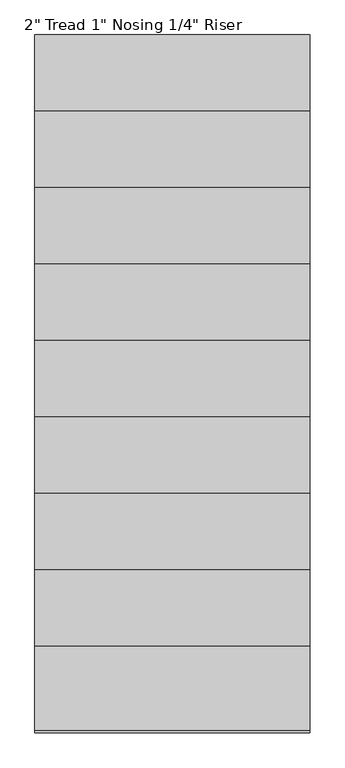
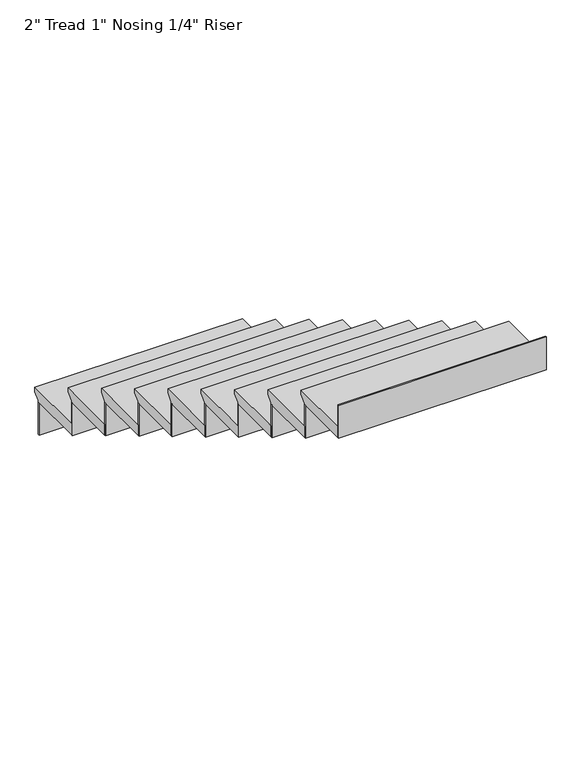
"""IFC4 building model written with IfcOpenShell, lengths in millimetres: stair flight geometry."""

from ifc_helpers import new_model, si_unit, frame, origin, place, context, project, spatial, polyline, outline, extrude, source, transform, mapped, element, save


def stair_flight_b6fb1fe0(model_context):
    return source(origin(), model_context, "Body", "SweptSolid", [
        extrude(outline(polyline([(-2919.1227897, 5029.2), (-2639.7227897, 5029.2), (-2639.7227897, 5010.15), (-2665.1227897, 4984.75), (-2665.1227897, 4978.4), (-2919.1227897, 4978.4), (-2919.1227897, 5029.2)])), frame((-9500.8771954, 0.0, 0.0), z_axis=(1.0, 0.0, 0.0), x_axis=(0.0, 1.0, 0.0)), (0.0, 0.0, 1.0), 914.4),
        extrude(outline(polyline([(-9500.8771954, -2671.4727897), (-9500.8771954, -2665.1227897), (-8586.4771954, -2665.1227897), (-8586.4771954, -2671.4727897), (-9500.8771954, -2671.4727897)])), frame((0.0, 0.0, 4826.0), z_axis=(0.0, 0.0, 1.0), x_axis=(1.0, 0.0, 0.0)), (0.0, 0.0, 1.0), 152.4),
        extrude(outline(polyline([(-9500.8771954, -2925.4727897), (-9500.8771954, -2919.1227897), (-8586.4771954, -2919.1227897), (-8586.4771954, -2925.4727897), (-9500.8771954, -2925.4727897)])), frame((0.0, 0.0, 4978.4), z_axis=(0.0, 0.0, 1.0), x_axis=(1.0, 0.0, 0.0)), (0.0, 0.0, 1.0), 152.4),
        extrude(outline(polyline([(-3173.1227897, 5181.6), (-2893.7227897, 5181.6), (-2893.7227897, 5162.55), (-2919.1227897, 5137.15), (-2919.1227897, 5130.8), (-3173.1227897, 5130.8), (-3173.1227897, 5181.6)])), frame((-9500.8771954, 0.0, 0.0), z_axis=(1.0, 0.0, 0.0), x_axis=(0.0, 1.0, 0.0)), (0.0, 0.0, 1.0), 914.4),
        extrude(outline(polyline([(-9500.8771954, -3179.4727897), (-9500.8771954, -3173.1227897), (-8586.4771954, -3173.1227897), (-8586.4771954, -3179.4727897), (-9500.8771954, -3179.4727897)])), frame((0.0, 0.0, 5130.8), z_axis=(0.0, 0.0, 1.0), x_axis=(1.0, 0.0, 0.0)), (0.0, 0.0, 1.0), 152.4),
        extrude(outline(polyline([(-3427.1227897, 5334.0), (-3147.7227897, 5334.0), (-3147.7227897, 5314.95), (-3173.1227897, 5289.55), (-3173.1227897, 5283.2), (-3427.1227897, 5283.2), (-3427.1227897, 5334.0)])), frame((-9500.8771954, 0.0, 0.0), z_axis=(1.0, 0.0, 0.0), x_axis=(0.0, 1.0, 0.0)), (0.0, 0.0, 1.0), 914.4),
        extrude(outline(polyline([(-9500.8771954, -3433.4727897), (-9500.8771954, -3427.1227897), (-8586.4771954, -3427.1227897), (-8586.4771954, -3433.4727897), (-9500.8771954, -3433.4727897)])), frame((0.0, 0.0, 5283.2), z_axis=(0.0, 0.0, 1.0), x_axis=(1.0, 0.0, 0.0)), (0.0, 0.0, 1.0), 152.4),
        extrude(outline(polyline([(-3681.1227897, 5486.4), (-3401.7227897, 5486.4), (-3401.7227897, 5467.35), (-3427.1227897, 5441.95), (-3427.1227897, 5435.6), (-3681.1227897, 5435.6), (-3681.1227897, 5486.4)])), frame((-9500.8771954, 0.0, 0.0), z_axis=(1.0, 0.0, 0.0), x_axis=(0.0, 1.0, 0.0)), (0.0, 0.0, 1.0), 914.4),
        extrude(outline(polyline([(-9500.8771954, -3687.4727897), (-9500.8771954, -3681.1227897), (-8586.4771954, -3681.1227897), (-8586.4771954, -3687.4727897), (-9500.8771954, -3687.4727897)])), frame((0.0, 0.0, 5435.6), z_axis=(0.0, 0.0, 1.0), x_axis=(1.0, 0.0, 0.0)), (0.0, 0.0, 1.0), 152.4),
        extrude(outline(polyline([(-3935.1227897, 5638.8), (-3655.7227897, 5638.8), (-3655.7227897, 5619.75), (-3681.1227897, 5594.35), (-3681.1227897, 5588.0), (-3935.1227897, 5588.0), (-3935.1227897, 5638.8)])), frame((-9500.8771954, 0.0, 0.0), z_axis=(1.0, 0.0, 0.0), x_axis=(0.0, 1.0, 0.0)), (0.0, 0.0, 1.0), 914.4),
        extrude(outline(polyline([(-9500.8771954, -3941.4727897), (-9500.8771954, -3935.1227897), (-8586.4771954, -3935.1227897), (-8586.4771954, -3941.4727897), (-9500.8771954, -3941.4727897)])), frame((0.0, 0.0, 5588.0), z_axis=(0.0, 0.0, 1.0), x_axis=(1.0, 0.0, 0.0)), (0.0, 0.0, 1.0), 152.4),
        extrude(outline(polyline([(-4189.1227897, 5791.2), (-3909.7227897, 5791.2), (-3909.7227897, 5772.15), (-3935.1227897, 5746.75), (-3935.1227897, 5740.4), (-4189.1227897, 5740.4), (-4189.1227897, 5791.2)])), frame((-9500.8771954, 0.0, 0.0), z_axis=(1.0, 0.0, 0.0), x_axis=(0.0, 1.0, 0.0)), (0.0, 0.0, 1.0), 914.4),
        extrude(outline(polyline([(-9500.8771954, -4195.4727897), (-9500.8771954, -4189.1227897), (-8586.4771954, -4189.1227897), (-8586.4771954, -4195.4727897), (-9500.8771954, -4195.4727897)])), frame((0.0, 0.0, 5740.4), z_axis=(0.0, 0.0, 1.0), x_axis=(1.0, 0.0, 0.0)), (0.0, 0.0, 1.0), 152.4),
        extrude(outline(polyline([(-4443.1227897, 5943.6), (-4163.7227897, 5943.6), (-4163.7227897, 5924.55), (-4189.1227897, 5899.15), (-4189.1227897, 5892.8), (-4443.1227897, 5892.8), (-4443.1227897, 5943.6)])), frame((-9500.8771954, 0.0, 0.0), z_axis=(1.0, 0.0, 0.0), x_axis=(0.0, 1.0, 0.0)), (0.0, 0.0, 1.0), 914.4),
        extrude(outline(polyline([(-9500.8771954, -4449.4727897), (-9500.8771954, -4443.1227897), (-8586.4771954, -4443.1227897), (-8586.4771954, -4449.4727897), (-9500.8771954, -4449.4727897)])), frame((0.0, 0.0, 5892.8), z_axis=(0.0, 0.0, 1.0), x_axis=(1.0, 0.0, 0.0)), (0.0, 0.0, 1.0), 152.4),
        extrude(outline(polyline([(-4697.1227897, 6096.0), (-4417.7227897, 6096.0), (-4417.7227897, 6076.95), (-4443.1227897, 6051.55), (-4443.1227897, 6045.2), (-4697.1227897, 6045.2), (-4697.1227897, 6096.0)])), frame((-9500.8771954, 0.0, 0.0), z_axis=(1.0, 0.0, 0.0), x_axis=(0.0, 1.0, 0.0)), (0.0, 0.0, 1.0), 914.4),
        extrude(outline(polyline([(-9500.8771954, -4703.4727897), (-9500.8771954, -4697.1227897), (-8586.4771954, -4697.1227897), (-8586.4771954, -4703.4727897), (-9500.8771954, -4703.4727897)])), frame((0.0, 0.0, 6045.2), z_axis=(0.0, 0.0, 1.0), x_axis=(1.0, 0.0, 0.0)), (0.0, 0.0, 1.0), 152.4),
        extrude(outline(polyline([(-9500.8771954, -4957.4727897), (-9500.8771954, -4951.1227897), (-8586.4771954, -4951.1227897), (-8586.4771954, -4957.4727897), (-9500.8771954, -4957.4727897)])), frame((0.0, 0.0, 6197.6), z_axis=(0.0, 0.0, 1.0), x_axis=(1.0, 0.0, 0.0)), (0.0, 0.0, 1.0), 152.4),
        extrude(outline(polyline([(-4951.1227897, 6248.4), (-4671.7227897, 6248.4), (-4671.7227897, 6229.35), (-4697.1227897, 6203.95), (-4697.1227897, 6197.6), (-4951.1227897, 6197.6), (-4951.1227897, 6248.4)])), frame((-9500.8771954, 0.0, 0.0), z_axis=(1.0, 0.0, 0.0), x_axis=(0.0, 1.0, 0.0)), (0.0, 0.0, 1.0), 914.4),
    ])


if __name__ == "__main__":
    model = new_model("IFC4")
    model_context = context("Model", 3, world=origin())
    ifc_project = project(units=[si_unit("LENGTHUNIT", "METRE", prefix="MILLI")], contexts=[model_context])
    site = spatial("IfcSite", under=ifc_project)
    building = spatial("IfcBuilding", under=site)
    placement = place(None, origin())
    stair_flight_shape = stair_flight_b6fb1fe0(model_context)
    element("IfcStairFlight", 1, ObjectType="2\" Tread 1\" Nosing 1/4\" Riser", at=placement, inside=building, context=model_context, shape_type="MappedRepresentation", body=[
        mapped(stair_flight_shape, transform((0.0, 0.0, 0.0), x_axis=(1.0, 0.0, 0.0), y_axis=(0.0, 1.0, 0.0), z_axis=(0.0, 0.0, 1.0))),
    ])
    save(model, "model.ifc")
